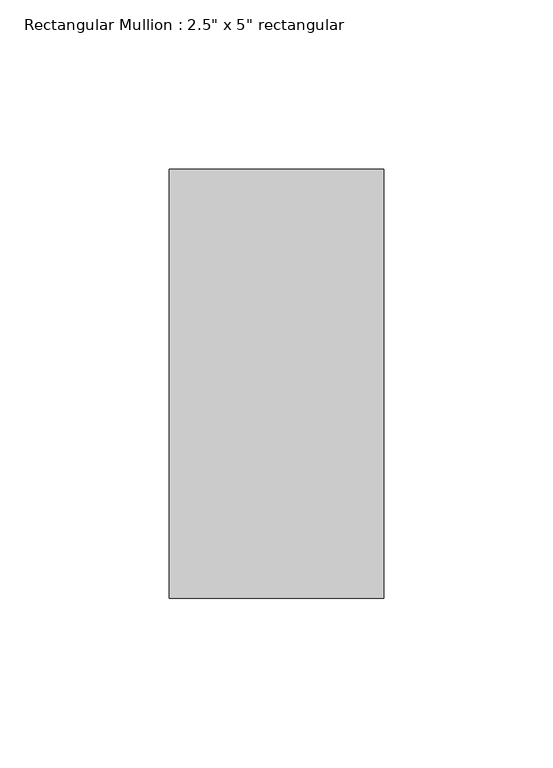
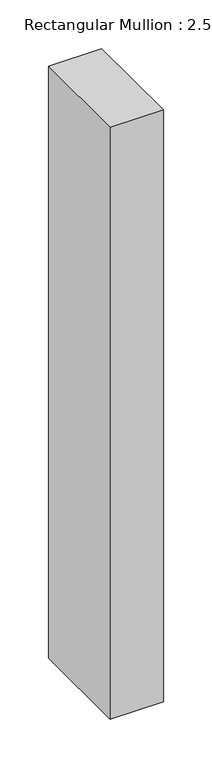
"""IFC4 building model written with IfcOpenShell, lengths in millimetres: member geometry."""

from ifc_helpers import new_model, si_unit, frame, origin, place, context, project, spatial, polyline, outline, extrude, source, transform, mapped, element, save


def member_0ce7375f(model_context):
    return source(origin(), model_context, "Body", "SweptSolid", [
        extrude(outline(polyline([(0.0, 63.5), (0.0, -63.5), (-63.5, -63.5), (-63.5, 63.5), (0.0, 63.5)])), frame((0.0, 0.0, -744.75), z_axis=(0.0, 0.0, 1.0), x_axis=(1.0, 0.0, 0.0)), (0.0, 0.0, 1.0), 744.75),
    ])


if __name__ == "__main__":
    model = new_model("IFC4")
    model_context = context("Model", 3, world=origin())
    ifc_project = project(units=[si_unit("LENGTHUNIT", "METRE", prefix="MILLI")], contexts=[model_context])
    site = spatial("IfcSite", under=ifc_project)
    building = spatial("IfcBuilding", under=site)
    placement = place(None, origin())
    member_shape = member_0ce7375f(model_context)
    element("IfcMember", 1, ObjectType="Rectangular Mullion : 2.5\" x 5\" rectangular", at=placement, inside=building, context=model_context, shape_type="MappedRepresentation", body=[
        mapped(member_shape, transform((0.0, 0.0, 0.0), x_axis=(1.0, 0.0, 0.0), y_axis=(0.0, 1.0, 0.0), z_axis=(0.0, 0.0, 1.0))),
    ])
    save(model, "model.ifc")

# Revit data of these elements
# Type "Rectangular Mullion : 2.5\" x 5\" rectangular"
#   built-in parameter 1007304 = 0.416667 (stored number, unit not read)
#   built-in parameter 1007301 = 0.104167 (stored number, unit not read)
#   built-in parameter 1007300 = 0.104167 (stored number, unit not read)
# Element 1 (IfcMember, "Rectangular Mullion : 2.5\" x 5\" rectangular")
#   Materials on its faces: "Damp-proofing"
# Materials
#   "Damp-proofing": class "Generic", colour RGB 127 127 127, transparency 0, Description = "Damp-proofing", Cost = 0
